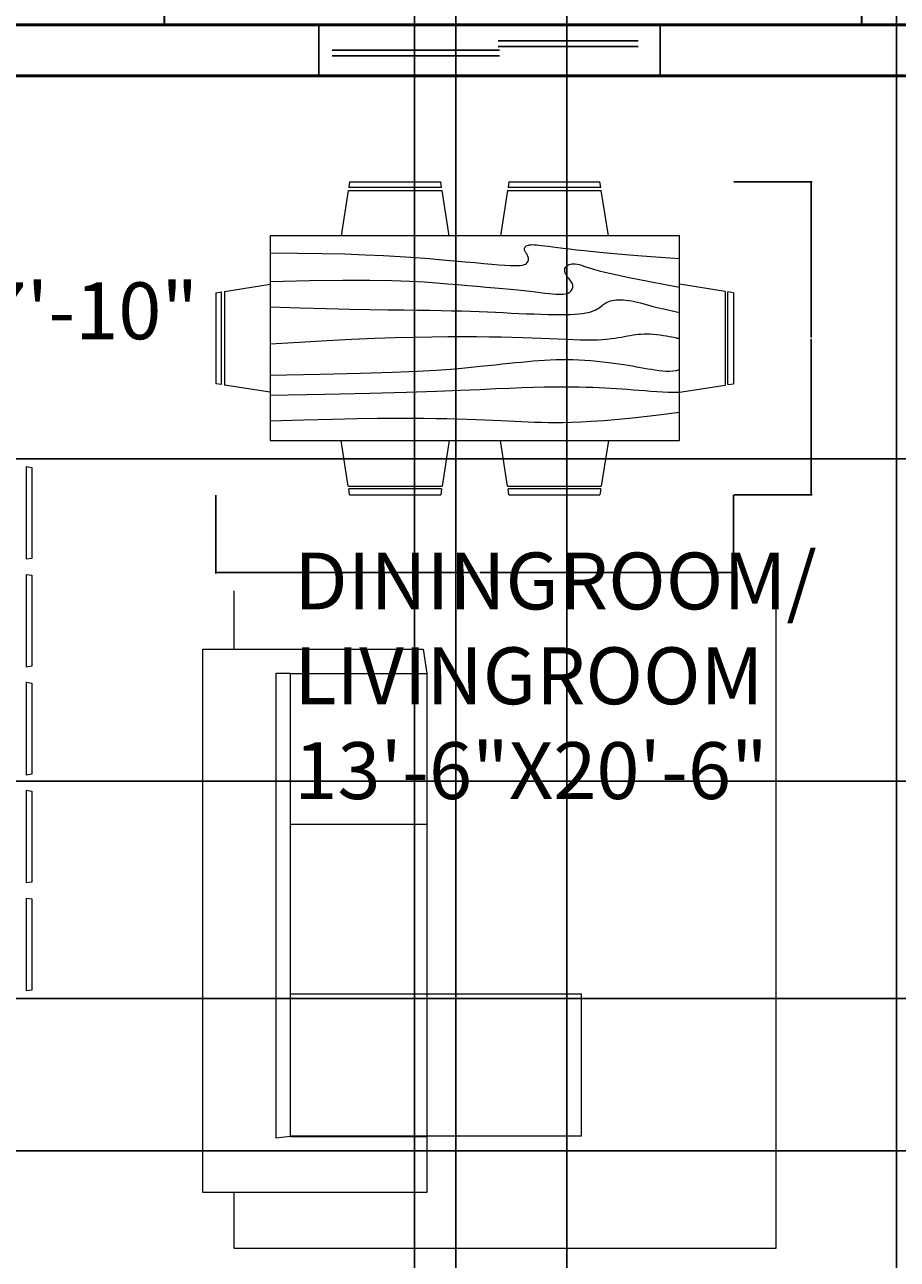
# Model space of a CAD drawing. Units: inches. Extents: x 821 to 2399, y 74 to 823.
# Tile 4 of 13: x 975 to 1128, y 381 to 599. Entities that reach past the tile are written whole.
import ezdxf

# ---------------------------------------------------------------- set-up
doc = ezdxf.new("R2010")
doc.units = ezdxf.units.IN
doc.header["$MEASUREMENT"] = 0
doc.layers.get('0').update_dxf_attribs({"lineweight": 53})
for name, color, linetype, lineweight in [('A-ANNO-DIMS', 2, 'Continuous', 18), ('A-AREA-IDEN', 7, 'Continuous', 18), ('A-DOOR', 4, 'Continuous', 25), ('A-FLOR', 7, 'Continuous', 30), ('A-FURN', 8, 'Continuous', 18), ('WALLS', 7, 'Continuous', 50)]:
    doc.layers.add(name, color=color, linetype=linetype, lineweight=lineweight)
doc.styles.get("Standard").update_dxf_attribs({"font": 'arial.ttf'})
doc.dimstyles.get("Standard").update_dxf_attribs({"dimtxt": 0.18, "dimasz": 0.18, "dimexe": 0.18, "dimexo": 0.0625, "dimgap": 0.09, "dimtad": 0, "dimtih": 1, "dimtoh": 1, "dimdec": 4, "dimzin": 0, "dimdsep": 46, "dimtxsty": 'Standard', "dimcen": 0.09, "dimadec": 0, "dimazin": 0, "dimtfac": 1, "dimtdec": 4, "dimtofl": 0, "dimtmove": 0, "dimatfit": 3, "dimfxl": 1, "dimtolj": 1, "dimtzin": 0, "dimarcsym": 0})

# ---------------------------------------------------------------- blocks, each defined once
blk = doc.blocks.new('Dining Set - 36 x 72 in.')
for p, q in [((-22, 27.5), (-22.1562, 26.50042)), ((-5.8416, 26.5), (-22.1534, 26.5)), ((-22, 27.5), (-6, 27.5)), ((-5.8437, 26.49966), (-6, 27.5)), ((6, 27.5), (5.8438, 26.50042)), ((22.1584, 26.5), (5.8466, 26.5)), ((6, 27.5), (22, 27.5)), ((22.1563, 26.49966), (22, 27.5)), ((-22.2343, 26.00059), (-23.4847, 17.99762)), ((-22.2304, 26), (-5.7608, 26)), ((-4.5152, 17.99762), (-5.7655, 25.99926)), ((5.7657, 26.00059), (4.5153, 17.99762)), ((5.7696, 26), (22.2392, 26)), ((23.4848, 17.99762), (22.2345, 25.99926)), ((36, 18), (-36, 18)), ((-36, 18), (-36, -18)), ((36, -18), (36, 18)), ((-44.0006, 8.23428), (-35.9976, 9.48474)), ((44.0006, 8.23428), (35.9976, 9.48474)), ((-45.5, 8), (-44.5004, 8.15617)), ((-45.5, 8), (-45.5, -8)), ((-44.5, -8.15843), (-44.5, 8.15338)), ((-44, 8.23041), (-44, -8.23915)), ((44, 8.23041), (44, -8.23915)), ((44.5, -8.15843), (44.5, 8.15338)), ((45.5, 8), (44.5005, 8.15617)), ((45.5, 8), (45.5, -8)), ((-44.4997, -8.15631), (-45.5, -8)), ((-35.9976, -9.48476), (-43.9993, -8.2345)), ((35.9976, -9.48476), (43.9993, -8.2345)), ((44.4997, -8.15631), (45.5, -8)), ((-36, -18), (36, -18)), ((-22.2343, -26.0006), (-23.4847, -17.99762)), ((-4.5152, -17.99762), (-5.7655, -25.99928)), ((5.7657, -26.0006), (4.5153, -17.99762)), ((23.4848, -17.99762), (22.2345, -25.99928)), ((-22.2304, -26), (-5.7608, -26)), ((5.7696, -26), (22.2392, -26)), ((-22, -27.5), (-22.1562, -26.50044)), ((-5.8416, -26.5), (-22.1534, -26.5)), ((-22, -27.5), (-6, -27.5)), ((-5.8437, -26.49967), (-6, -27.5)), ((6, -27.5), (5.8438, -26.50044)), ((22.1584, -26.5), (5.8466, -26.5)), ((6, -27.5), (22, -27.5)), ((22.1563, -26.49967), (22, -27.5))]:
    blk.add_line(p, q)
for points in [[(-36, 15), (-31.1772, 14.97754), (-26.8079, 14.91406), (-22.8538, 14.81543), (-19.276, 14.6875), (-16.0362, 14.53613), (-13.0957, 14.36718), (-10.4159, 14.18652), (-7.9583, 14), (-5.6904, 13.81315), (-3.6035, 13.63021), (-1.6954, 13.45508), (0.0365, 13.29166), (1.5945, 13.14388), (2.9811, 13.01562), (4.1988, 12.9108), (5.25, 12.83333), (6.1393, 12.78613), (6.8802, 12.76823), (7.4883, 12.77767), (7.9792, 12.8125), (8.3685, 12.87077), (8.6719, 12.95052), (8.9049, 13.0498), (9.0833, 13.16666), (9.2205, 13.29899), (9.3216, 13.44401), (9.3895, 13.59879), (9.4271, 13.76041), (9.4373, 13.92594), (9.4232, 14.09245), (9.3875, 14.257), (9.3333, 14.41666), (9.2638, 14.56917), (9.1836, 14.71484), (9.0975, 14.85465), (9.0104, 14.98958), (8.9272, 15.1206), (8.8529, 15.2487), (8.7922, 15.37483), (8.75, 15.5), (8.7305, 15.62467), (8.7344, 15.74739), (8.7617, 15.86621), (8.8125, 15.97916), (8.8867, 16.08431), (8.9844, 16.17968), (9.1055, 16.26334), (9.25, 16.33333), (9.4189, 16.38802), (9.6172, 16.42708), (9.8506, 16.45052), (10.125, 16.45833), (10.4463, 16.45052), (10.8203, 16.42708), (11.2529, 16.38802), (11.75, 16.33333), (12.3184, 16.26318), (12.9694, 16.17838), (13.7151, 16.07991), (14.5677, 15.96875), (15.5395, 15.84586), (16.6426, 15.71224), (17.8893, 15.56884), (19.2917, 15.41666), (20.859, 15.25667), (22.5879, 15.08984), (24.4721, 14.91715), (26.5052, 14.73958), (28.6809, 14.5581), (30.9929, 14.3737), (33.4347, 14.18733), (36, 14)], [(-36, 10), (-28.9766, 10.14274), (-23.1725, 10.20442), (-18.4241, 10.19775), (-14.5677, 10.13541), (-11.4399, 10.03011), (-8.877, 9.89453), (-6.7154, 9.74137), (-4.7917, 9.58333), (-2.9698, 9.43082), (-1.2246, 9.28515), (0.4415, 9.14534), (2.026, 9.01041), (3.5266, 8.87939), (4.9408, 8.7513), (6.266, 8.62516), (7.5, 8.5), (8.6411, 8.37549), (9.6914, 8.2539), (10.6538, 8.13818), (11.5312, 8.03125), (12.3267, 7.93603), (13.043, 7.85547), (13.6831, 7.79248), (14.25, 7.75), (14.7471, 7.7303), (15.1797, 7.73307), (15.5537, 7.75732), (15.875, 7.80208), (16.1494, 7.86637), (16.3828, 7.94922), (16.5811, 8.04964), (16.75, 8.16666), (16.8944, 8.29915), (17.0143, 8.44531), (17.1089, 8.60319), (17.1771, 8.77083), (17.218, 8.94629), (17.2305, 9.1276), (17.2137, 9.31282), (17.1667, 9.5), (17.0895, 9.6875), (16.987, 9.875), (16.8649, 10.0625), (16.7292, 10.25), (16.5856, 10.4375), (16.4401, 10.625), (16.2985, 10.8125), (16.1667, 11), (16.05, 11.18733), (15.9518, 11.3737), (15.8752, 11.5581), (15.8229, 11.73958), (15.798, 11.91715), (15.8034, 12.08984), (15.842, 12.25667), (15.9167, 12.41666), (16.0295, 12.56836), (16.1784, 12.70833), (16.3605, 12.83268), (16.5729, 12.9375), (16.8127, 13.01888), (17.0768, 13.07291), (17.3625, 13.0957), (17.6667, 13.08333), (17.9894, 13.03312), (18.3418, 12.94726), (18.7382, 12.82918), (19.1927, 12.68229), (19.7195, 12.51001), (20.3327, 12.31575), (21.0465, 12.10294), (21.875, 11.875), (22.8357, 11.63354), (23.959, 11.37304), (25.2786, 11.08618), (26.8282, 10.76562), (28.6414, 10.40405), (30.752, 9.99414), (33.1936, 9.52856), (36, 9)], [(-36, 5.5), (-30.7157, 5.3348), (-26.069, 5.20963), (-21.9946, 5.11767), (-18.4271, 5.05208), (-15.3009, 5.00602), (-12.5508, 4.97265), (-10.1112, 4.94515), (-7.9167, 4.91666), (-5.909, 4.88167), (-4.0586, 4.83984), (-2.3429, 4.79215), (-0.7396, 4.73958), (0.7739, 4.6831), (2.22, 4.6237), (3.6213, 4.56233), (5, 4.5), (6.373, 4.43782), (7.7344, 4.3776), (9.0723, 4.32129), (10.375, 4.27083), (11.6309, 4.22819), (12.8281, 4.19531), (13.9551, 4.17415), (15, 4.16666), (15.954, 4.17448), (16.819, 4.19791), (17.6001, 4.23698), (18.3021, 4.29166), (18.9299, 4.36198), (19.4883, 4.44791), (19.9823, 4.54948), (20.4167, 4.66666), (20.7969, 4.79899), (21.1302, 4.94401), (21.4245, 5.09879), (21.6875, 5.26041), (21.9271, 5.42594), (22.1511, 5.59245), (22.3672, 5.757), (22.5834, 5.91666), (22.8065, 6.06868), (23.0404, 6.21093), (23.2879, 6.34147), (23.5521, 6.45833), (23.8358, 6.55957), (24.142, 6.64323), (24.4735, 6.70735), (24.8334, 6.75), (25.2235, 6.76969), (25.642, 6.76692), (26.0858, 6.74267), (26.5521, 6.69791), (27.0379, 6.63362), (27.5404, 6.55078), (28.0565, 6.45036), (28.5834, 6.33333), (29.1242, 6.19987), (29.7071, 6.04687), (30.3661, 5.87044), (31.1354, 5.66666), (32.0493, 5.43164), (33.142, 5.16146), (34.4475, 4.85221), (36, 4.5)], [(-36, -1), (-30.7915, -0.6591), (-26.0195, -0.38216), (-21.6519, -0.16284), (-17.6563, 0.00521), (-14.0005, 0.12833), (-10.6523, 0.21289), (-7.5796, 0.26522), (-4.75, 0.29166), (-2.134, 0.29793), (0.2878, 0.28711), (2.5317, 0.26163), (4.6146, 0.22396), (6.5529, 0.17651), (8.3633, 0.12174), (10.0623, 0.06209), (11.6667, 0), (13.1899, -0.06201), (14.6341, -0.1211), (15.9982, -0.17432), (17.2813, -0.21875), (18.4823, -0.25147), (19.6003, -0.26953), (20.6343, -0.27002), (21.5834, -0.25), (22.4481, -0.20768), (23.2357, -0.14584), (23.9549, -0.06836), (24.6146, 0.02083), (25.2235, 0.11784), (25.7904, 0.21875), (26.3241, 0.31966), (26.8334, 0.41666), (27.3265, 0.50618), (27.8099, 0.58593), (28.2894, 0.65397), (28.7709, 0.70833), (29.2601, 0.74707), (29.763, 0.76823), (30.2855, 0.76985), (30.8334, 0.75), (31.4088, 0.70784), (31.9994, 0.64713), (32.589, 0.57275), (33.1615, 0.48958), (33.7008, 0.4025), (34.1908, 0.3164), (34.6153, 0.23616), (34.9584, 0.16666), (35.2099, 0.11165), (35.3848, 0.07031), (35.504, 0.04069), (35.5886, 0.02083), (35.6594, 0.00879), (35.7377, 0.0026), (35.8442, 0.00032), (36, 0)], [(-36, -6.5), (-27.1843, -6.31267), (-20.084, -6.1263), (-14.469, -5.9419), (-10.1094, -5.76042), (-6.7752, -5.58285), (-4.2363, -5.41016), (-2.2629, -5.24333), (-0.625, -5.08334), (0.8708, -4.93099), (2.2715, -4.78646), (3.5872, -4.64974), (4.8281, -4.52084), (6.0046, -4.39974), (7.127, -4.28646), (8.2053, -4.18099), (9.25, -4.08334), (10.2705, -3.99382), (11.2734, -3.91407), (12.2647, -3.84603), (13.25, -3.79167), (14.2354, -3.75293), (15.2266, -3.73177), (16.2295, -3.73015), (17.25, -3.75), (18.2912, -3.79248), (19.3451, -3.85547), (20.4009, -3.93604), (21.4479, -4.03125), (22.4754, -4.13819), (23.4727, -4.25391), (24.4289, -4.37549), (25.3334, -4.5), (26.1785, -4.62492), (26.9694, -4.74935), (27.7145, -4.87281), (28.4219, -4.99479), (29.1, -5.11483), (29.7572, -5.23242), (30.4016, -5.34709), (31.0417, -5.45834), (31.6837, -5.56437), (32.3262, -5.65821), (32.9658, -5.73153), (33.599, -5.77604), (34.2224, -5.78345), (34.8327, -5.74545), (35.4264, -5.65373), (36, -5.5)], [(-36, -10), (-26.4022, -9.81299), (-18.4675, -9.62891), (-11.9839, -9.45069), (-6.7396, -9.28125), (-2.5226, -9.12354), (0.8789, -8.98047), (3.6769, -8.85498), (6.0833, -8.75), (8.2767, -8.66765), (10.3021, -8.60677), (12.1712, -8.56543), (13.8958, -8.54167), (15.4876, -8.53353), (16.9583, -8.53907), (18.3197, -8.55632), (19.5834, -8.58334), (20.7616, -8.61841), (21.8685, -8.66081), (22.9188, -8.71004), (23.9271, -8.76563), (24.9081, -8.82707), (25.8763, -8.89388), (26.8465, -8.96558), (27.8334, -9.04167), (28.8474, -9.12118), (29.8828, -9.20117), (30.93, -9.27824), (31.9792, -9.34896), (33.0205, -9.40991), (34.0443, -9.45768), (35.0407, -9.48885), (36, -9.5)], [(-36, -14.5), (-30.0881, -14.33513), (-25.0332, -14.21224), (-20.7312, -14.12647), (-17.0781, -14.07292), (-13.97, -14.04671), (-11.3027, -14.04297), (-8.9724, -14.05681), (-6.875, -14.08334), (-4.9224, -14.11833), (-3.0905, -14.16016), (-1.3709, -14.20785), (0.2448, -14.26042), (1.7647, -14.3169), (3.1973, -14.3763), (4.5507, -14.43767), (5.8333, -14.5), (7.0554, -14.5621), (8.235, -14.62175), (9.3922, -14.67652), (10.5469, -14.72396), (11.7192, -14.76164), (12.929, -14.78711), (14.1965, -14.79794), (15.5417, -14.79167), (16.9933, -14.76424), (18.6152, -14.70508), (20.4804, -14.60197), (22.6615, -14.44271), (25.2312, -14.21509), (28.2624, -13.9069), (31.8277, -13.50594), (36, -13)]]:
    blk.add_lwpolyline(points)
blk = doc.blocks.new('*D50')
at = {"layer": 'A-ANNO-DIMS', "color": 0, "lineweight": -2, "transparency": 16777216}
for p, q in [((1008.48, 515.83), (1008.48, 502.06)), ((1099.48, 515.83), (1099.48, 502.06)), ((1008.66, 502.24), (1053.03, 502.24)), ((1099.3, 502.24), (1054.93, 502.24))]:
    blk.add_line(p, q, dxfattribs=at)
at = {"layer": 'A-ANNO-DIMS', "color": 0, "lineweight": 50, "transparency": 16777216}
for points in [[(1008.66, 502.27), (1008.66, 502.21), (1008.48, 502.24)], [(1099.3, 502.27), (1099.3, 502.21), (1099.48, 502.24)]]:
    blk.add_solid(points, dxfattribs=at)
at = {"layer": 'Defpoints', "color": 0, "lineweight": 50, "transparency": 16777216}
for p in [(1008.48, 515.89), (1099.48, 515.89), (1099.48, 502.24)]:
    blk.add_point(p, dxfattribs=at)
at = {"layer": 'A-ANNO-DIMS', "color": 0, "transparency": 16777216, "insert": (1053.98, 502.24), "char_height": 0.18, "attachment_point": 5}
blk.add_mtext('\\A1;DINING SET 91', dxfattribs=at)
blk = doc.blocks.new('*D51')
at = {"layer": 'A-ANNO-DIMS', "color": 0, "lineweight": -2, "transparency": 16777216}
for p, q in [((1099.54, 570.89), (1113.31, 570.89)), ((1113.13, 570.71), (1113.13, 543.58)), ((1113.13, 516.07), (1113.13, 543.21)), ((1099.54, 515.89), (1113.31, 515.89))]:
    blk.add_line(p, q, dxfattribs=at)
at = {"layer": 'A-ANNO-DIMS', "color": 0, "lineweight": 50, "transparency": 16777216}
for points in [[(1113.1, 570.71), (1113.16, 570.71), (1113.13, 570.89)], [(1113.1, 516.07), (1113.16, 516.07), (1113.13, 515.89)]]:
    blk.add_solid(points, dxfattribs=at)
at = {"layer": 'Defpoints', "color": 0, "lineweight": 50, "transparency": 16777216}
for p in [(1099.48, 570.89), (1113.13, 570.89), (1099.48, 515.89)]:
    blk.add_point(p, dxfattribs=at)
at = {"layer": 'A-ANNO-DIMS', "color": 0, "transparency": 16777216, "insert": (1113.13, 543.39), "char_height": 0.18, "attachment_point": 5}
blk.add_mtext('\\A1;55', dxfattribs=at)
blk = doc.blocks.new('*D80')
at = {"layer": 'A-ANNO-DIMS', "color": 0, "lineweight": -2, "transparency": 16777216}
for p, q in [((999.33, 754.12), (820.74, 754.12)), ((820.92, 753.94), (820.92, 430.67)), ((820.92, 107.04), (820.92, 430.31)), ((1050.58, 106.86), (820.74, 106.86))]:
    blk.add_line(p, q, dxfattribs=at)
at = {"layer": 'A-ANNO-DIMS', "color": 0, "lineweight": 50, "transparency": 16777216}
for points in [[(820.89, 753.94), (820.95, 753.94), (820.92, 754.12)], [(820.89, 107.04), (820.95, 107.04), (820.92, 106.86)]]:
    blk.add_solid(points, dxfattribs=at)
at = {"layer": 'Defpoints', "color": 0, "lineweight": 50, "transparency": 16777216}
for p in [(999.39, 754.12), (820.92, 106.86), (1050.64, 106.86)]:
    blk.add_point(p, dxfattribs=at)
at = {"layer": 'A-ANNO-DIMS', "color": 0, "transparency": 16777216, "insert": (820.92, 430.49), "char_height": 0.18, "attachment_point": 5}
blk.add_mtext('\\A1;647.3', dxfattribs=at)
blk = doc.blocks.new('*D81')
at = {"layer": 'A-ANNO-DIMS', "color": 0, "lineweight": -2, "transparency": 16777216}
for p, q in [((853.37, 292.61), (853.37, 786.75)), ((853.55, 786.57), (948.09, 786.57)), ((1043.19, 786.57), (948.65, 786.57)), ((1043.37, 292.58), (1043.37, 786.75))]:
    blk.add_line(p, q, dxfattribs=at)
at = {"layer": 'A-ANNO-DIMS', "color": 0, "lineweight": 50, "transparency": 16777216}
for points in [[(853.55, 786.6), (853.55, 786.54), (853.37, 786.57)], [(1043.19, 786.6), (1043.19, 786.54), (1043.37, 786.57)]]:
    blk.add_solid(points, dxfattribs=at)
at = {"layer": 'Defpoints', "color": 0, "lineweight": 50, "transparency": 16777216}
for p in [(1043.37, 786.57), (853.37, 292.55), (1043.37, 292.52)]:
    blk.add_point(p, dxfattribs=at)
at = {"layer": 'A-ANNO-DIMS', "color": 0, "transparency": 16777216, "insert": (948.37, 786.57), "char_height": 0.18, "attachment_point": 5}
blk.add_mtext('\\A1;190', dxfattribs=at)
blk = doc.blocks.new('*D89')
at = {"layer": 'A-ANNO-DIMS', "color": 0, "lineweight": -2, "transparency": 16777216}
for p, q in [((1050.64, 106.93), (1050.64, 786.75)), ((1050.82, 786.57), (1088.99, 786.57)), ((1127.94, 786.57), (1089.78, 786.57)), ((1128.12, 106.93), (1128.12, 786.75))]:
    blk.add_line(p, q, dxfattribs=at)
at = {"layer": 'A-ANNO-DIMS', "color": 0, "lineweight": 50, "transparency": 16777216}
for points in [[(1050.82, 786.6), (1050.82, 786.54), (1050.64, 786.57)], [(1127.94, 786.6), (1127.94, 786.54), (1128.12, 786.57)]]:
    blk.add_solid(points, dxfattribs=at)
at = {"layer": 'Defpoints', "color": 0, "lineweight": 50, "transparency": 16777216}
for p in [(1128.12, 786.57), (1050.64, 106.86), (1128.12, 106.86)]:
    blk.add_point(p, dxfattribs=at)
at = {"layer": 'A-ANNO-DIMS', "color": 0, "transparency": 16777216, "insert": (1089.38, 786.57), "char_height": 0.18, "attachment_point": 5}
blk.add_mtext('\\A1;77.48', dxfattribs=at)
blk = doc.blocks.new('*D91')
at = {"layer": 'A-ANNO-DIMS', "color": 0, "lineweight": -2, "transparency": 16777216}
for p, q in [((1043.37, 200.58), (1043.37, 786.75)), ((1043.55, 786.57), (1056.29, 786.57)), ((1069.96, 786.57), (1057.22, 786.57)), ((1070.14, 200.58), (1070.14, 786.75))]:
    blk.add_line(p, q, dxfattribs=at)
at = {"layer": 'A-ANNO-DIMS', "color": 0, "lineweight": 50, "transparency": 16777216}
for points in [[(1043.55, 786.6), (1043.55, 786.54), (1043.37, 786.57)], [(1069.96, 786.6), (1069.96, 786.54), (1070.14, 786.57)]]:
    blk.add_solid(points, dxfattribs=at)
at = {"layer": 'Defpoints', "color": 0, "lineweight": 50, "transparency": 16777216}
for p in [(1070.14, 786.57), (1043.37, 200.52), (1070.14, 200.52)]:
    blk.add_point(p, dxfattribs=at)
at = {"layer": 'A-ANNO-DIMS', "color": 0, "transparency": 16777216, "insert": (1056.75, 786.57), "char_height": 0.18, "attachment_point": 5}
blk.add_mtext('\\A1;26.763', dxfattribs=at)
blk = doc.blocks.new('*D97')
at = {"layer": 'A-ANNO-DIMS', "color": 0, "lineweight": -2, "transparency": 16777216}
for p, q in [((1152.31, 465.52), (820.74, 465.52)), ((820.92, 465.34), (820.92, 433.2)), ((820.92, 400.7), (820.92, 432.84)), ((1152.31, 400.52), (820.74, 400.52))]:
    blk.add_line(p, q, dxfattribs=at)
at = {"layer": 'A-ANNO-DIMS', "color": 0, "lineweight": 50, "transparency": 16777216}
for points in [[(820.89, 465.34), (820.95, 465.34), (820.92, 465.52)], [(820.89, 400.7), (820.95, 400.7), (820.92, 400.52)]]:
    blk.add_solid(points, dxfattribs=at)
at = {"layer": 'Defpoints', "color": 0, "lineweight": 50, "transparency": 16777216}
for p in [(820.92, 465.52), (1152.37, 465.52), (1152.37, 400.52)]:
    blk.add_point(p, dxfattribs=at)
at = {"layer": 'A-ANNO-DIMS', "color": 0, "transparency": 16777216, "insert": (820.92, 433.02), "char_height": 0.18, "attachment_point": 5}
blk.add_mtext('\\A1;65', dxfattribs=at)
blk = doc.blocks.new('*D103')
at = {"layer": 'A-ANNO-DIMS', "color": 0, "lineweight": -2, "transparency": 16777216}
for p, q in [((966.67, 522.18), (1330, 522.18)), ((1329.82, 522), (1329.82, 474.94)), ((1329.82, 427.51), (1329.82, 474.57)), ((966.67, 427.33), (1330, 427.33))]:
    blk.add_line(p, q, dxfattribs=at)
at = {"layer": 'A-ANNO-DIMS', "color": 0, "lineweight": 50, "transparency": 16777216}
for points in [[(1329.79, 522), (1329.85, 522), (1329.82, 522.18)], [(1329.79, 427.51), (1329.85, 427.51), (1329.82, 427.33)]]:
    blk.add_solid(points, dxfattribs=at)
at = {"layer": 'Defpoints', "color": 0, "lineweight": 50, "transparency": 16777216}
for p in [(966.61, 522.18), (1329.82, 522.18), (966.61, 427.33)]:
    blk.add_point(p, dxfattribs=at)
at = {"layer": 'A-ANNO-DIMS', "color": 0, "transparency": 16777216, "insert": (1329.82, 474.75), "char_height": 0.18, "attachment_point": 5}
blk.add_mtext('\\A1;94.85', dxfattribs=at)

msp = doc.modelspace()

# ---------------------------------------------------------------- linework, layer by layer
at = {"layer": 'A-DOOR'}
for p, q in [((1058.0986, 595.7078), (1082.6824, 595.7078)), ((1028.9323, 594.0195), (1058.3418, 594.0195)), ((1028.9323, 593.0195), (1058.3418, 593.0195)), ((1058.0986, 594.7078), (1082.6824, 594.7078))]:
    msp.add_line(p, q, dxfattribs=at)
msp.add_lwpolyline([(1086.564, 589.5195), (1086.564, 598.5195), (1026.564, 598.5195), (1026.564, 589.5195)], close=True, dxfattribs=at)
at = {"layer": 'A-FLOR'}
msp.add_lwpolyline([(1122.0283, 598.5195), (1122.0283, 669.4726), (1048.7194, 669.4726), (1048.7194, 754.1164), (999.3938, 754.1164), (999.3938, 598.5195)], dxfattribs=at)
at = {"layer": 'A-FURN'}
for p, q in [((975.1131, 520.8505), (975.1131, 504.5387)), ((975.1131, 501.881), (975.1131, 485.5692)), ((1021.5655, 484.4651), (1018.9875, 484.4651)), ((1018.9875, 484.4651), (1018.9875, 402.8316)), ((975.1131, 482.9115), (975.1131, 466.5997)), ((975.1131, 463.942), (975.1131, 447.6302)), ((1021.5655, 457.9516), (1045.5757, 457.9516)), ((975.1131, 444.9725), (975.1131, 428.6607)), ((1018.9875, 402.8316), (1021.5655, 403.1142))]:
    msp.add_line(p, q, dxfattribs=at)
for points in [[(975.1128, 520.8484), (976.1131, 520.6921), (976.1131, 504.6921), (975.1135, 504.5359)], [(975.1128, 501.8789), (976.1131, 501.7226), (976.1131, 485.7226), (975.1135, 485.5664)], [(1106.9128, 498.9878), (1106.9128, 383.3743), (1011.676, 383.3743), (1011.676, 393.1928)], [(1011.676, 488.7426), (1011.676, 498.9878)], [(1045.5757, 403.0088), (1045.5757, 393.1928), (1006.1792, 393.1928), (1006.1792, 488.7426), (1044.877, 488.7426), (1045.5757, 484.4651)], [(975.1128, 482.9094), (976.1131, 482.7531), (976.1131, 466.7531), (975.1135, 466.5969)], [(975.1128, 463.9399), (976.1131, 463.7836), (976.1131, 447.7836), (975.1135, 447.6274)], [(975.1128, 444.9704), (976.1131, 444.8141), (976.1131, 428.8141), (975.1135, 428.6579)]]:
    msp.add_lwpolyline(points, dxfattribs=at)
for points in [[(1021.5655, 484.4651), (1045.5757, 484.4651), (1045.5757, 403.0088), (1021.5655, 403.0088)], [(1021.5655, 428.1152), (1072.7056, 428.1152), (1072.7056, 403.1142), (1021.5655, 403.1142)]]:
    msp.add_lwpolyline(points, close=True, dxfattribs=at)
at = {"layer": 'WALLS'}
msp.add_lwpolyline([(1050.641, 200.5195), (1050.641, 170.9407), (1121.9086, 170.9407), (1128.124, 170.9407), (1050.641, 170.9407), (1050.641, 106.8645), (1128.124, 106.8645), (1128.124, 170.9407), (1128.124, 200.5195), (1288.3735, 200.5195), (1297.3735, 200.5195), (1297.3735, 598.5195), (853.3735, 598.5195), (853.3735, 292.549), (922.3673, 292.5195), (1043.3735, 292.5195), (1043.3735, 209.5195), (1043.3735, 200.5195)], close=True, dxfattribs=at)
msp.add_lwpolyline([(862.3735, 589.5195), (1148.3735, 589.5195), (1148.3735, 563.3933), (1148.3735, 565.3933), (1150.3735, 565.3933), (1150.3735, 563.3933), (1174.3735, 563.3933)], dxfattribs=at)

# ---------------------------------------------------------------- block references
at = {"layer": 'A-FURN'}
msp.add_blockref('Dining Set - 36 x 72 in.', (1053.9825, 543.3939), dxfattribs=at)

# ---------------------------------------------------------------- texts
at = {"layer": 'A-AREA-IDEN', "char_height": 10, "attachment_point": 1}
for s, width, insert in [('KITCHEN\\P10\'-6"X17\'-10"', 75.475047, (914.5519, 569.8843)), ('DININGROOM/\\PLIVINGROOM\\P13\'-6"X20\'-6"', 94.426507, (1022.258, 505.7225))]:
    msp.add_mtext_dynamic_manual_height_columns(s, width=width, gutter_width=1, heights=[0], dxfattribs=dict(at, insert=insert))

# ---------------------------------------------------------------- dimensions: what is measured, and where the dimension line sits
at = {"layer": 'A-ANNO-DIMS'}
for base, p1, p2, override, picture, middle in [((1043.3735, 786.5664), (853.3735, 292.549), (1043.3735, 292.5195), {"dimdec": 0, "dimlfac": 1, "dimrnd": 0, "dimzin": 0, "dimdsep": 46, "dimlunit": 2}, '*D81', (948.3735, 786.5664)), ((1070.1365, 786.5664), (1043.3735, 200.5195), (1070.1365, 200.5195), {"dimdec": 3, "dimlfac": 1, "dimrnd": 0, "dimzin": 0, "dimdsep": 46, "dimlunit": 2}, '*D91', (1056.755, 786.5664)), ((1128.124, 786.5664), (1050.641, 106.8645), (1128.124, 106.8645), {"dimdec": 2, "dimlfac": 1, "dimrnd": 0, "dimzin": 0, "dimdsep": 46, "dimlunit": 2}, '*D89', (1089.3825, 786.5664))]:
    dim = msp.add_linear_dim(base=base, p1=p1, p2=p2, dimstyle='Standard', override=override, dxfattribs=at)
    dim.commit()
    dim.dimension.update_dxf_attribs({"geometry": picture, "text_midpoint": middle})
for base, p1, p2, override, picture, middle in [((820.9235, 106.8645), (999.3938, 754.1164), (1050.641, 106.8645), {"dimdec": 1, "dimlfac": 1, "dimrnd": 0, "dimzin": 0, "dimdsep": 46, "dimlunit": 2}, '*D80', (820.9235, 430.4905)), ((1113.1325, 570.8939), (1099.4825, 515.8939), (1099.4825, 570.8939), {"dimdec": 0, "dimlfac": 1, "dimrnd": 0, "dimzin": 0, "dimdsep": 46, "dimlunit": 2}, '*D51', (1113.1325, 543.3939)), ((1329.8235, 522.1769), (966.6107, 427.3294), (966.6107, 522.1769), {"dimdec": 2, "dimlfac": 1, "dimrnd": 0, "dimzin": 0, "dimdsep": 46, "dimlunit": 2}, '*D103', (1329.8235, 474.7531)), ((820.9235, 465.5195), (1152.3735, 400.5195), (1152.3735, 465.5195), {"dimdec": 0, "dimlfac": 1, "dimrnd": 0, "dimzin": 0, "dimdsep": 46, "dimlunit": 2}, '*D97', (820.9235, 433.0195))]:
    dim = msp.add_linear_dim(base=base, p1=p1, p2=p2, angle=90, dimstyle='Standard', override=override, dxfattribs=at)
    dim.commit()
    dim.dimension.update_dxf_attribs({"geometry": picture, "text_midpoint": middle})
dim = msp.add_linear_dim(base=(1099.4825, 502.2439), p1=(1008.4825, 515.8939), p2=(1099.4825, 515.8939), text='DINING SET <>', dimstyle='Standard', override={"dimdec": 0, "dimlfac": 1, "dimrnd": 0, "dimzin": 0, "dimdsep": 46, "dimlunit": 2}, dxfattribs=at)
dim.commit()
dim.dimension.update_dxf_attribs({"geometry": '*D50', "text_midpoint": (1053.9825, 502.2439)})

doc.saveas('drawing.dxf')
